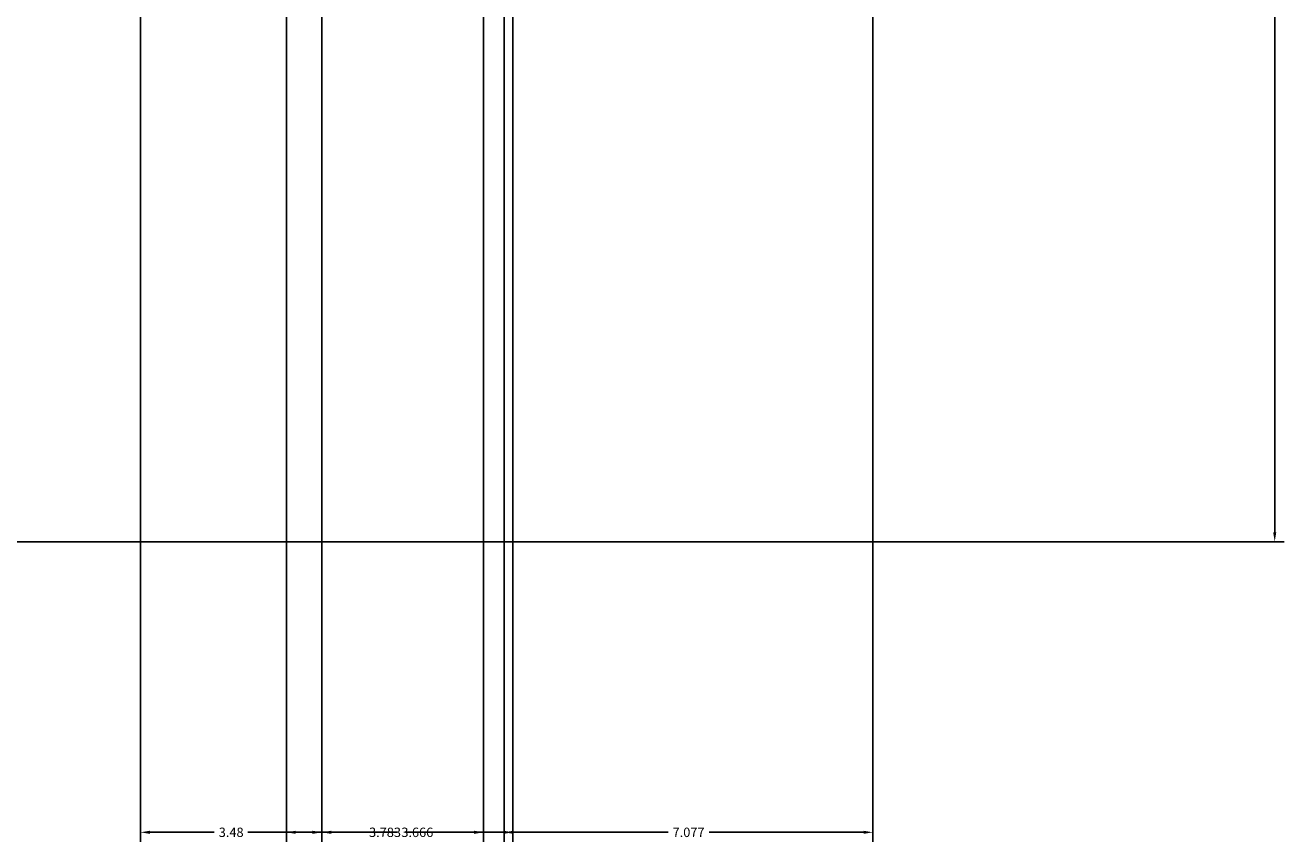
# Model space of a CAD drawing. Units: inches. Extents: x 23 to 132, y 5 to 105.
# Tile 8 of 14: x 105 to 129, y 5 to 21. Entities that reach past the tile are written whole.
import ezdxf

# ---------------------------------------------------------------- set-up
doc = ezdxf.new("R2010")
doc.units = ezdxf.units.IN
doc.header["$MEASUREMENT"] = 0
doc.layers.add('A-ANNO-DIMS', color=2, linetype='Continuous', lineweight=18)
doc.styles.get("Standard").update_dxf_attribs({"font": 'arial.ttf'})
doc.dimstyles.get("Standard").update_dxf_attribs({"dimtxt": 0.18, "dimasz": 0.18, "dimexe": 0.18, "dimexo": 0.0625, "dimgap": 0.09, "dimtad": 0, "dimtih": 1, "dimtoh": 1, "dimdec": 4, "dimzin": 0, "dimdsep": 46, "dimtxsty": 'Standard', "dimcen": 0.09, "dimadec": 0, "dimazin": 0, "dimtfac": 1, "dimtdec": 4, "dimtofl": 0, "dimtmove": 0, "dimatfit": 3, "dimfxl": 1, "dimtolj": 1, "dimtzin": 0, "dimarcsym": 0})

# ---------------------------------------------------------------- blocks, each defined once
blk = doc.blocks.new('*D3')
at = {"layer": 'A-ANNO-DIMS', "color": 0, "lineweight": -2, "transparency": 16777216}
for p, q in [((121.409, 99.285), (129.239, 99.285)), ((129.059, 99.105), (129.059, 55.423)), ((129.059, 11.378), (129.059, 55.06)), ((72.981, 11.198), (129.239, 11.198))]:
    blk.add_line(p, q, dxfattribs=at)
at = {"layer": 'A-ANNO-DIMS', "color": 0, "transparency": 16777216}
for points in [[(129.029, 99.105), (129.089, 99.105), (129.059, 99.285)], [(129.029, 11.378), (129.089, 11.378), (129.059, 11.198)]]:
    blk.add_solid(points, dxfattribs=at)
at = {"layer": 'Defpoints', "color": 0, "transparency": 16777216}
for p in [(121.346, 99.285), (129.059, 99.285), (72.919, 11.198)]:
    blk.add_point(p, dxfattribs=at)
at = {"layer": 'A-ANNO-DIMS', "color": 0, "transparency": 16777216, "insert": (129.059, 55.241), "char_height": 0.18, "attachment_point": 5}
blk.add_mtext('\\A1;88.09', dxfattribs=at)
blk = doc.blocks.new('*D75')
at = {"layer": 'A-ANNO-DIMS', "color": 0, "lineweight": -2, "transparency": 16777216}
for p, q in [((107.287, 59.528), (107.287, 5.443)), ((110.768, 59.503), (110.768, 5.443)), ((107.467, 5.623), (108.704, 5.623)), ((110.588, 5.623), (109.351, 5.623))]:
    blk.add_line(p, q, dxfattribs=at)
at = {"layer": 'A-ANNO-DIMS', "color": 0, "transparency": 16777216}
for points in [[(107.467, 5.653), (107.467, 5.593), (107.287, 5.623)], [(110.588, 5.653), (110.588, 5.593), (110.768, 5.623)]]:
    blk.add_solid(points, dxfattribs=at)
at = {"layer": 'Defpoints', "color": 0, "transparency": 16777216}
for p in [(107.287, 59.59), (110.768, 59.566), (110.768, 5.623)]:
    blk.add_point(p, dxfattribs=at)
at = {"layer": 'A-ANNO-DIMS', "color": 0, "transparency": 16777216, "insert": (109.028, 5.623), "char_height": 0.18, "attachment_point": 5}
blk.add_mtext('\\A1;3.48', dxfattribs=at)
blk = doc.blocks.new('*D76')
at = {"layer": 'A-ANNO-DIMS', "color": 0, "lineweight": -2, "transparency": 16777216}
for p, q in [((114.434, 59.528), (114.434, 5.443)), ((110.768, 59.503), (110.768, 5.443)), ((110.948, 5.623), (112.207, 5.623)), ((114.254, 5.623), (112.994, 5.623))]:
    blk.add_line(p, q, dxfattribs=at)
at = {"layer": 'A-ANNO-DIMS', "color": 0, "transparency": 16777216}
for points in [[(110.948, 5.653), (110.948, 5.593), (110.768, 5.623)], [(114.254, 5.653), (114.254, 5.593), (114.434, 5.623)]]:
    blk.add_solid(points, dxfattribs=at)
at = {"layer": 'Defpoints', "color": 0, "transparency": 16777216}
for p in [(110.768, 59.566), (114.434, 59.59), (114.434, 5.623)]:
    blk.add_point(p, dxfattribs=at)
at = {"layer": 'A-ANNO-DIMS', "color": 0, "transparency": 16777216, "insert": (112.601, 5.623), "char_height": 0.18, "attachment_point": 5}
blk.add_mtext('\\A1;3.666', dxfattribs=at)
blk = doc.blocks.new('*D91')
at = {"layer": 'A-ANNO-DIMS', "color": 0, "lineweight": -2, "transparency": 16777216}
for p, q in [((110.089, 79.853), (110.089, 5.443)), ((113.872, 79.853), (113.872, 5.443)), ((110.269, 5.623), (111.587, 5.623)), ((113.692, 5.623), (112.374, 5.623))]:
    blk.add_line(p, q, dxfattribs=at)
at = {"layer": 'A-ANNO-DIMS', "color": 0, "transparency": 16777216}
for points in [[(110.269, 5.653), (110.269, 5.593), (110.089, 5.623)], [(113.692, 5.653), (113.692, 5.593), (113.872, 5.623)]]:
    blk.add_solid(points, dxfattribs=at)
at = {"layer": 'Defpoints', "color": 0, "transparency": 16777216}
for p in [(110.089, 79.916), (113.872, 79.916), (113.872, 5.623)]:
    blk.add_point(p, dxfattribs=at)
at = {"layer": 'A-ANNO-DIMS', "color": 0, "transparency": 16777216, "insert": (111.981, 5.623), "char_height": 0.18, "attachment_point": 5}
blk.add_mtext('\\A1;3.783', dxfattribs=at)
blk = doc.blocks.new('*D93')
at = {"layer": 'A-ANNO-DIMS', "color": 0, "lineweight": -2, "transparency": 16777216}
for p, q in [((114.269, 94.721), (114.269, 5.443)), ((121.346, 94.721), (121.346, 5.443)), ((114.449, 5.623), (117.415, 5.623)), ((121.166, 5.623), (118.201, 5.623))]:
    blk.add_line(p, q, dxfattribs=at)
at = {"layer": 'A-ANNO-DIMS', "color": 0, "transparency": 16777216}
for points in [[(114.449, 5.653), (114.449, 5.593), (114.269, 5.623)], [(121.166, 5.653), (121.166, 5.593), (121.346, 5.623)]]:
    blk.add_solid(points, dxfattribs=at)
at = {"layer": 'Defpoints', "color": 0, "transparency": 16777216}
for p in [(114.269, 94.783), (121.346, 94.783), (121.346, 5.623)]:
    blk.add_point(p, dxfattribs=at)
at = {"layer": 'A-ANNO-DIMS', "color": 0, "transparency": 16777216, "insert": (117.808, 5.623), "char_height": 0.18, "attachment_point": 5}
blk.add_mtext('\\A1;7.077', dxfattribs=at)

msp = doc.modelspace()

# ---------------------------------------------------------------- dimensions: what is measured, and where the dimension line sits
at = {"layer": 'A-ANNO-DIMS'}
dim = msp.add_linear_dim(base=(129.0589, 99.2846), p1=(72.9188, 11.1983), p2=(121.3461, 99.2846), angle=90, dimstyle='Standard', override={"dimdec": 2, "dimlfac": 1, "dimrnd": 0, "dimzin": 0, "dimdsep": 46, "dimlunit": 2}, dxfattribs=at)
dim.commit()
dim.dimension.update_dxf_attribs({"geometry": '*D3', "text_midpoint": (129.0589, 55.2415)})
for base, p1, p2, override, picture, middle in [((121.3461, 5.6233), (114.2693, 94.7833), (121.3461, 94.7833), {"dimdec": 3, "dimlfac": 1, "dimrnd": 0, "dimzin": 0, "dimdsep": 46, "dimlunit": 2}, '*D93', (117.8077, 5.6233)), ((113.8719, 5.6233), (110.0892, 79.9158), (113.8719, 79.9158), {"dimdec": 3, "dimlfac": 1, "dimrnd": 0, "dimzin": 0, "dimdsep": 46, "dimlunit": 2}, '*D91', (111.9805, 5.6233)), ((110.7677, 5.6233), (107.2874, 59.5904), (110.7677, 59.566), {"dimdec": 2, "dimlfac": 1, "dimrnd": 0, "dimzin": 0, "dimdsep": 46, "dimlunit": 2}, '*D75', (109.0275, 5.6233)), ((114.434, 5.6233), (110.7677, 59.566), (114.434, 59.5904), {"dimdec": 3, "dimlfac": 1, "dimrnd": 0, "dimzin": 0, "dimdsep": 46, "dimlunit": 2}, '*D76', (112.6009, 5.6233))]:
    dim = msp.add_linear_dim(base=base, p1=p1, p2=p2, dimstyle='Standard', override=override, dxfattribs=at)
    dim.commit()
    dim.dimension.update_dxf_attribs({"geometry": picture, "text_midpoint": middle})

doc.saveas('drawing.dxf')
